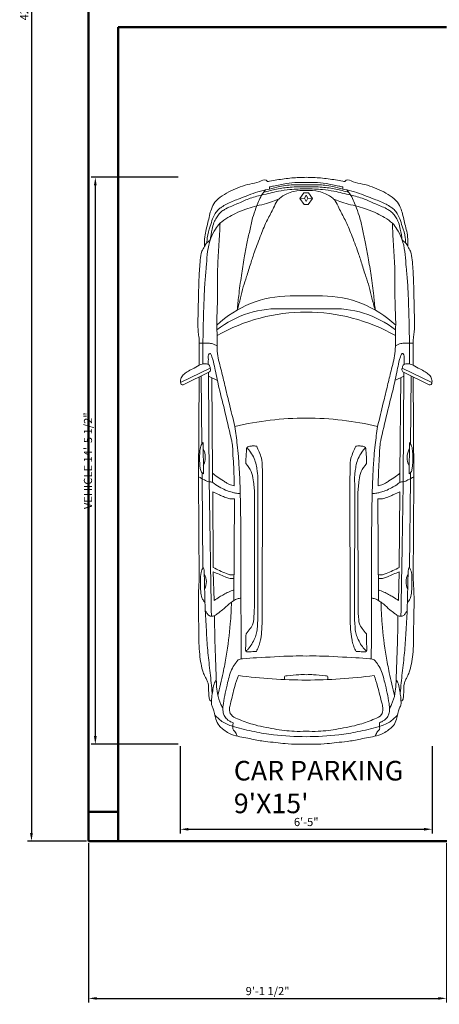
# Model space of a CAD drawing. Units: inches. Extents: x 20697 to 21575, y 6189 to 6822.
# Tile 1 of 7: x 20697 to 20826, y 6189 to 6490. Entities that reach past the tile are written whole.
import ezdxf

# ---------------------------------------------------------------- set-up
doc = ezdxf.new("R2010")
doc.units = ezdxf.units.IN
for name, color, linetype, lineweight in [('A-ANNO-DIMS', 2, 'Continuous', 18), ('A-AREA-IDEN', 7, 'Continuous', 18), ('A-SITE-VEHC', 8, 'Continuous', 13), ('A-WALL', 7, 'Continuous', 50)]:
    doc.layers.add(name, color=color, linetype=linetype, lineweight=lineweight)
doc.styles.get("Standard").update_dxf_attribs({"font": 'arial.ttf'})
doc.dimstyles.new('ISO-25', dxfattribs={"dimtxt": 2.5, "dimasz": 2.5, "dimexe": 1.25, "dimexo": 0.625, "dimtad": 1, "dimdec": 0, "dimlunit": 3, "dimtxsty": 'Standard', "dimcen": 2.5, "dimadec": 0, "dimazin": 0, "dimtfac": 1, "dimtdec": 0, "dimtmove": 0, "dimatfit": 3, "dimfxl": 1, "dimarcsym": 0})

# ---------------------------------------------------------------- blocks, each defined once
blk = doc.blocks.new('*D6')
at = {"layer": 'A-ANNO-DIMS', "color": 0, "lineweight": -2, "transparency": 16777216}
for p, q in [((20717.67, 6750.06), (20699.54, 6750.06)), ((20700.79, 6747.56), (20700.79, 6241.06)), ((20717.67, 6238.56), (20699.54, 6238.56))]:
    blk.add_line(p, q, dxfattribs=at)
at = {"layer": 'A-ANNO-DIMS', "color": 0, "transparency": 16777216}
for points in [[(20700.37, 6747.56), (20701.21, 6747.56), (20700.79, 6750.06)], [(20700.37, 6241.06), (20701.21, 6241.06), (20700.79, 6238.56)]]:
    blk.add_solid(points, dxfattribs=at)
at = {"layer": 'Defpoints', "color": 0, "transparency": 16777216}
for p in [(20718.29, 6750.06), (20700.79, 6238.56), (20718.29, 6238.56)]:
    blk.add_point(p, dxfattribs=at)
at = {"layer": 'A-ANNO-DIMS', "color": 0, "transparency": 16777216, "insert": (20698.89, 6494.31), "char_height": 2.5, "attachment_point": 5, "rotation": 90}
blk.add_mtext('42\'-8"', dxfattribs=at)
blk = doc.blocks.new('A$C37D034A9')
for p, q in [((1532.9, 1782), (1646.8, 2021.3)), ((1562, 1787.5), (1667.1, 1999.6)), ((1303.4, 1869.8), (1509.9, 1870.9)), ((1332.7, 1840.6), (1499.3, 1841.7)), ((1594.8, 1853.7), (2145, 1849.8)), ((1603.5, 1871.3), (2420.8, 1875.4)), ((2129.3, 1839.6), (2381.5, 1836.9)), ((2373.8, 1848.2), (2422.4, 1847.8)), ((2420.8, 1875.4), (3234.3, 1871.4)), ((2422.4, 1847.8), (3133.1, 1841.3)), ((3158, 1831.3), (3479.6, 1822.1)), ((1565.9, 1795.4), (2445.8, 1790.4)), ((1632.4, 1724.1), (1596.5, 1795.2)), ((2377.3, 1763.7), (1609.3, 1769.9)), ((2377.3, 1763.7), (2449.6, 1763.3)), ((2525, 1762.2), (3132.5, 1759)), ((3168.1, 1757.9), (3399.7, 1751.2)), ((2582.7, 1587), (3399.6, 1592.9)), ((2539.6, 1425.8), (3453, 1427.6)), ((2405.7, 1362.6), (3533.3, 1364.3)), ((2458.8, 1400.3), (3499.1, 1398.6)), ((76.9, 1306.3), (96.6, 1306.3)), ((96.6, 1306.3), (101.3, 1337.1)), ((952, 1010.8), (952, 1141.1)), ((1057.1, 1010.8), (1057.1, 1185.6)), ((124.1, 1010.8), (124.7, 1029.9)), ((124.7, 1029.9), (169.4, 1060.8)), ((169.4, 1060.8), (168.8, 1024.8)), ((169.4, 1060.8), (219.8, 1027.6)), ((124.1, 1010.8), (124.7, 991.8)), ((124.7, 991.8), (169.4, 960.9)), ((143, 1010.8), (168.8, 1024.8)), ((143, 1010.8), (168.8, 996.9)), ((168.8, 1024.8), (195.2, 1010.8)), ((168.8, 996.9), (195.2, 1010.8)), ((169.4, 960.9), (168.8, 996.9)), ((169.4, 960.9), (219.8, 994.1)), ((219.8, 1027.6), (219.8, 1010.8)), ((219.8, 994.1), (219.8, 1010.8)), ((952, 1010.8), (952, 880.6)), ((1057.1, 1010.8), (1057.1, 836.1)), ((76.9, 715.4), (96.6, 715.4)), ((96.6, 715.4), (101.3, 684.5)), ((2405.7, 659.1), (3533.3, 657.4)), ((2458.8, 621.4), (3499.1, 623.1)), ((2539.6, 595.9), (3453, 594.1)), ((2582.7, 434.7), (3399.6, 428.8)), ((1532.9, 239.7), (1646.8, 0.4)), ((1632.4, 297.6), (1596.5, 226.5)), ((2377.3, 258), (1609.3, 251.8)), ((2377.3, 258), (2449.6, 258.4)), ((2525, 259.5), (3132.5, 262.7)), ((3168.1, 263.8), (3399.7, 270.5)), ((1332.7, 181), (1499.3, 180)), ((1562, 234.2), (1667.1, 22.1)), ((1565.9, 226.3), (2445.8, 231.3)), ((1594.8, 168), (2145, 171.9)), ((2129.3, 182.1), (2381.5, 184.7)), ((2373.8, 173.5), (2422.4, 173.9)), ((2422.4, 173.9), (3133.1, 180.4)), ((3158, 190.4), (3479.6, 199.6)), ((1303.4, 151.9), (1509.9, 150.8)), ((1603.5, 150.4), (2420.8, 146.3)), ((2420.8, 146.3), (3234.3, 150.3))]:
    blk.add_line(p, q)
for centre, radius, start, end in [((2249.9, 1966.9), 145.3, 241.65089, 297.15378), ((3250.7, 1930.2), 117.1, 238.4977, 298.20211), ((1820.6, 1134.2), 868.6, 136.71033, 179.54402), ((1853.1, 1235.9), 797.6, 141.87926, 183.61449), ((2543.6, 1010.3), 1461.1, 150.60457, 179.97848), ((4391.3, 1012.9), 2457.7, 166.55485, 180.04792), ((-73, 1011.6), 4110.5, 359.98923, 7.61333), ((2543.6, 1011.4), 1461.1, 180.02152, 209.39543), ((4391.3, 1008.8), 2457.7, 179.95208, 193.44515), ((-73, 1010.1), 4110.5, 352.38667, 0.01077), ((1820.6, 887.5), 868.6, 180.45598, 223.28967), ((1853.1, 785.8), 797.6, 176.38551, 218.12074), ((2249.9, 54.7), 145.3, 62.84622, 118.34911), ((3250.7, 91.5), 117.1, 61.79789, 121.5023)]:
    blk.add_arc(centre, radius, start, end)
for points, knots in [([(1526.7, 1783.8), (1518.5, 1785.4), (1502.6, 1788.6), (1494, 1821.1), (1503, 1863.1), (1531.4, 1908.3), (1553.6, 1954.9), (1577.5, 1992.7), (1609, 2018.2), (1639.6, 2023.8), (1665.5, 2017.7), (1667.4, 2005.2), (1667.1, 1999.6)], [0, 0, 0, 0, 0.0238674, 0.0459576, 0.0928721, 0.1559652, 0.2092168, 0.2528802, 0.29396, 0.3295755, 0.3493177, 0.3652101, 0.3652101, 0.3652101, 0.3652101]), ([(0, 1010.8), (0.9, 1049.4), (2.7, 1128.2), (18.7, 1227.6), (27.1, 1289.4), (36.3, 1321.4), (9.1, 1341.9), (46.5, 1397.5), (51.1, 1463.8), (76, 1541.9), (106.6, 1616.4), (147, 1685.7), (193.4, 1744.6), (269.5, 1782.5), (364.9, 1798.9), (463.9, 1829.1), (529.8, 1828.6), (556.4, 1828.4)], [0, 0, 0, 0, 115.859327, 237.079713, 296.141984, 312.044705, 327.106088, 383.833978, 461.944264, 541.76825, 623.45364, 704.555207, 782.226587, 843.70687, 954.283591, 1071.961262, 1151.295838, 1151.295838, 1151.295838, 1151.295838]), ([(171.7, 1228.4), (179.9, 1245.7), (198.1, 1284.1), (217.3, 1351.6), (232.9, 1424.6), (256.4, 1502.6), (284.7, 1575), (325.4, 1642.9), (361.7, 1702.7), (421.9, 1744.6), (473.5, 1772.8), (542.2, 1795.2), (621.2, 1808), (729.6, 1813.6), (852.5, 1827.6), (985.4, 1831.9), (1147.8, 1837.9), (1262.1, 1839.6), (1332.7, 1840.6)], [0, 0, 0, 0, 57.118397, 127.539793, 209.532187, 281.268626, 371.866644, 441.418243, 519.229725, 578.070076, 658.62539, 694.988053, 794.237238, 897.694875, 1020.566778, 1165.110139, 1296.310821, 1508.108184, 1508.108184, 1508.108184, 1508.108184]), ([(505.9, 1783.2), (511.7, 1792.2), (524.3, 1811.9), (558.6, 1828.8), (601.3, 1855.8), (687.8, 1865.5), (801.6, 1872.4), (931.7, 1876.4), (1052.9, 1878.6), (1152.2, 1881.4), (1229.2, 1880.7), (1271.8, 1874.5), (1295.8, 1871.8), (1303.4, 1869.8)], [0, 0, 0, 0, 0.0326993, 0.0711104, 0.1154542, 0.1883548, 0.3342533, 0.4716751, 0.5906313, 0.709353, 0.7812775, 0.8251283, 0.8483376, 0.8483376, 0.8483376, 0.8483376]), ([(1352.2, 1727.5), (1348.6, 1734.7), (1341.5, 1749.1), (1334, 1774.3), (1330.6, 1801.2), (1331.6, 1824.1), (1333.2, 1846.5), (1333.1, 1860.1), (1333, 1869.8)], [0, 0, 0, 0, 24.224889, 47.981341, 78.378061, 105.14947, 116.640041, 145.779732, 145.779732, 145.779732, 145.779732]), ([(2129.3, 1839.6), (2139.3, 1846.4), (2162.1, 1861.8), (2229.8, 1868.5), (2295.3, 1869), (2349.6, 1860.8), (2371.7, 1853), (2377.9, 1842.9), (2381.5, 1836.9)], [0, 0, 0, 0, 35.825501, 81.320865, 199.176406, 232.541501, 246.984194, 267.031211, 267.031211, 267.031211, 267.031211]), ([(2539.5, 1541.1), (2539.2, 1554), (2538.6, 1576.3), (2528.3, 1611.8), (2517, 1652), (2491.9, 1699.9), (2471, 1739.2), (2444.9, 1765.9), (2448.6, 1796.4), (2428.8, 1832.5), (2413.3, 1859.8), (2404.6, 1875.3)], [0, 0, 0, 0, 38.745445, 66.586145, 110.33194, 163.856449, 227.516292, 245.160425, 271.043315, 311.933858, 365.718129, 365.718129, 365.718129, 365.718129]), ([(3133.1, 1841.3), (3146.7, 1846.9), (3179.9, 1860.4), (3247.3, 1860.4), (3314.2, 1860.4), (3370.1, 1853.2), (3398.7, 1838.7), (3410.3, 1828.3), (3415.2, 1823.9)], [0, 0, 0, 0, 43.951201, 106.610136, 198.707081, 246.448273, 273.585601, 293.13086, 293.13086, 293.13086, 293.13086]), ([(3133.1, 1841.3), (3135, 1839.5), (3139.3, 1835.5), (3148, 1831.9), (3154.6, 1831.5), (3158, 1831.3)], [0, 0, 0, 0, 7.956866, 17.272723, 27.586643, 27.586643, 27.586643, 27.586643]), ([(3234.3, 1871.4), (3278.5, 1873.9), (3359.8, 1878.7), (3498.2, 1876.9), (3652.8, 1872.6), (3796.5, 1873.5), (3904.8, 1856.8), (3965.7, 1843.6), (4008.7, 1824.5), (4036.7, 1808.6), (4079.2, 1792.4), (4128.2, 1796.5), (4172.2, 1791.8), (4202.5, 1788.4), (4205.6, 1775.1), (4206.3, 1771.9)], [0, 0, 0, 0, 132.674859, 244.267951, 415.033268, 597.210204, 673.623963, 743.864874, 783.070086, 814.193218, 840.469708, 918.651615, 953.206586, 982.809878, 992.270601, 992.270601, 992.270601, 992.270601]), ([(3379.8, 1535.3), (3380.7, 1545.1), (3382.7, 1565.9), (3401.9, 1597.3), (3430.4, 1638), (3469.9, 1676.8), (3498.2, 1716.6), (3521, 1743.8), (3525.9, 1769.6), (3522.3, 1795.4), (3500.7, 1808.9), (3486.5, 1817.7), (3479.6, 1822.1)], [0, 0, 0, 0, 29.359586, 61.637967, 108.210927, 179.145324, 226.057178, 255.76704, 283.158676, 303.178471, 328.962154, 354.067963, 354.067963, 354.067963, 354.067963]), ([(3479.6, 1822.1), (3538.8, 1818.8), (3651.5, 1812.5), (3818.6, 1802.2), (3979.7, 1781.5), (4087.9, 1771.6), (4142.1, 1766.6)], [0, 0, 0, 0, 177.941766, 338.827113, 501.856877, 665.021059, 665.021059, 665.021059, 665.021059]), ([(101.3, 1337.1), (107.8, 1364.5), (120.6, 1417.6), (150.6, 1489.5), (178.2, 1568.8), (207.7, 1635.1), (236.1, 1688.4), (260.7, 1718.9), (292, 1744.4), (337.6, 1766.1), (403.7, 1784.8), (466.8, 1807.4), (512, 1808.2), (525.1, 1808.4)], [0, 0, 0, 0, 84.171622, 163.614553, 233.045723, 336.213067, 381.194856, 413.584235, 453.241792, 501.082694, 563.744046, 659.867603, 698.986252, 698.986252, 698.986252, 698.986252]), ([(142.1, 1367.1), (151.1, 1402.9), (168, 1470.3), (214.3, 1562.8), (239.3, 1634.9), (268.9, 1683.6), (292.1, 1711.1), (325.5, 1734.1), (365.7, 1755.6), (427.7, 1769.9), (475.9, 1778.1), (505.9, 1783.2)], [0, 0, 0, 0, 110.301969, 207.85498, 309.529413, 337.706505, 378.588004, 416.258758, 458.790096, 514.345906, 605.771135, 605.771135, 605.771135, 605.771135]), ([(1500.6, 1799.3), (1483.6, 1797.8), (1458.3, 1795.7), (1428.9, 1799.6), (1404, 1781.1), (1466.2, 1759.6), (1531.4, 1744.8), (1686.1, 1714.1), (1872.2, 1665.2), (2027.8, 1629.7), (2149.6, 1601.2), (2228.7, 1601.2), (2331, 1591.7), (2412.2, 1590.6), (2462.2, 1589.4), (2477.9, 1589.1)], [0, 0, 0, 0, 50.83029, 75.434549, 89.950931, 122.622478, 199.812772, 348.247849, 559.911218, 792.840685, 822.965183, 934.929309, 1028.100235, 1131.331462, 1178.338034, 1178.338034, 1178.338034, 1178.338034]), ([(1562, 1787.5), (1559.1, 1784.6), (1548.4, 1777.2), (1535.5, 1781.2), (1526.6, 1783.9)], [0.60973338, 0.60973338, 0.60973338, 0.60973338, 0.62203277, 0.64851229, 0.64851229, 0.64851229, 0.64851229]), ([(2477.9, 1589.1), (2475, 1602.1), (2470.4, 1622.6), (2455.4, 1651.1), (2432.7, 1682.8), (2408.1, 1722.8), (2386.6, 1751.4), (2377.3, 1763.7)], [0, 0, 0, 0, 39.93807, 62.488042, 96.043823, 157.027531, 203.188279, 203.188279, 203.188279, 203.188279]), ([(2445.8, 1790.4), (2667.6, 1786.9), (3027.2, 1781.3), (3386.8, 1774.8), (3524.6, 1772.4)], [0, 0, 0, 0, 665.499287, 1078.912831, 1078.912831, 1078.912831, 1078.912831]), ([(2582.7, 1587), (2583.2, 1597), (2584.1, 1618.1), (2575.7, 1651.7), (2561.4, 1682.9), (2545.4, 1721), (2533, 1746.1), (2525, 1762.2)], [0, 0, 0, 0, 29.813022, 63.072982, 102.549857, 133.014078, 186.71332, 186.71332, 186.71332, 186.71332]), ([(3190.5, 1591.4), (3191.8, 1602.2), (3194.2, 1623.2), (3178.9, 1661.6), (3159.5, 1706.6), (3141.5, 1741.5), (3132.5, 1759)], [0, 0, 0, 0, 32.129278, 62.428148, 121.529201, 180.173044, 180.173044, 180.173044, 180.173044]), ([(3221.3, 1591.6), (3222.3, 1599.2), (3224.2, 1612.8), (3218.1, 1637.1), (3198.8, 1684.5), (3181.3, 1726.4), (3168.1, 1757.9)], [0, 0, 0, 0, 22.895094, 40.749622, 74.16608, 176.695684, 176.695684, 176.695684, 176.695684]), ([(3399.7, 1751.2), (3389.2, 1737.2), (3370.8, 1712.4), (3351.4, 1671.7), (3328.3, 1635.1), (3318.4, 1607), (3313.2, 1592.2)], [0, 0, 0, 0, 52.277284, 92.404872, 134.765704, 181.565756, 181.565756, 181.565756, 181.565756]), ([(3520.4, 1748.4), (3581.5, 1747.4), (3690.9, 1745.6), (3850.5, 1740.6), (3997.8, 1733.6), (4128.7, 1732.6), (4218, 1705.9), (4256.1, 1686.1), (4266.8, 1680.5)], [0, 0, 0, 0, 0.1893068, 0.338908, 0.4944806, 0.646686, 0.7418914, 0.7794792, 0.7794792, 0.7794792, 0.7794792]), ([(4034.2, 1733.6), (4045.8, 1740.2), (4074.3, 1756.4), (4123, 1760.8), (4168.2, 1770.9), (4204, 1771), (4235.2, 1775.6), (4280.4, 1748.5), (4340.7, 1743.1), (4401.4, 1717.8), (4431.8, 1679.8), (4465, 1638.3), (4492.9, 1557.6), (4508.3, 1454.7), (4532.6, 1348.3), (4538.1, 1258.3), (4550, 1171.3), (4553.1, 1089.6), (4552.8, 1033), (4552.7, 1010.8)], [0, 0, 0, 0, 39.653141, 97.537887, 144.067219, 178.030901, 205.682198, 235.219107, 329.899318, 386.728403, 425.383384, 473.826134, 545.717065, 677.079425, 786.867362, 871.982002, 947.184951, 1050.283917, 1116.835862, 1116.835862, 1116.835862, 1116.835862]), ([(4319.3, 1743.9), (4339.8, 1723.4), (4383.7, 1679.5), (4421.6, 1566.1), (4452, 1430.6), (4487, 1238.2), (4490.2, 1098.7), (4492.3, 1010.8)], [0, 0, 0, 0, 85.725408, 184.11518, 350.578699, 505.359156, 768.57646, 768.57646, 768.57646, 768.57646]), ([(368.8, 1703.1), (425.1, 1705.7), (540.8, 1711), (717, 1724.8), (900.9, 1721.8), (1058.4, 1725.6), (1167.5, 1731.4), (1251.8, 1726.5), (1327.3, 1728.4), (1438.6, 1725.6), (1547.2, 1692.8), (1679.5, 1663), (1828.2, 1626.4), (1937.8, 1599.7), (2000.9, 1584.4)], [0, 0, 0, 0, 169.036427, 347.362971, 529.912023, 720.398665, 820.073141, 857.414524, 973.264583, 1046.863942, 1190.103596, 1310.627442, 1454.37964, 1649.234994, 1649.234994, 1649.234994, 1649.234994]), ([(3411.7, 1610.9), (3469.8, 1613.6), (3614.8, 1620.2), (3804, 1644.2), (3995.7, 1680.7), (4101, 1706), (4162.1, 1720.6)], [0, 0, 0, 0, 174.545563, 435.159645, 571.339835, 759.876078, 759.876078, 759.876078, 759.876078]), ([(4380.1, 1598.9), (4377.5, 1605.6), (4372, 1620.1), (4356.9, 1644.3), (4333.4, 1666.4), (4303.5, 1677.7), (4268.1, 1682), (4185.7, 1672.3), (4075, 1646.1), (3959.1, 1618.7), (3904, 1580.2), (3870.2, 1557), (3862, 1494.9), (3857.6, 1352), (3843.1, 1179.6), (3844.2, 1046.6), (3844.5, 1010.8)], [0, 0, 0, 0, 21.644576, 46.330939, 85.252079, 115.796407, 140.70863, 191.639103, 362.713195, 485.636819, 539.797523, 566.31637, 603.271258, 715.496747, 1007.274347, 1114.772665, 1114.772665, 1114.772665, 1114.772665]), ([(2000.9, 1584.4), (2050.2, 1577.5), (2130.3, 1566.4), (2257.3, 1554.3), (2428.3, 1543.9), (2677.9, 1536.6), (3173.5, 1535.9), (3575.5, 1534.8), (3868.2, 1533.9)], [0, 0, 0, 0, 149.160554, 242.516206, 382.750296, 663.136182, 991.365177, 1869.419131, 1869.419131, 1869.419131, 1869.419131]), ([(4001.2, 1556.2), (4030.1, 1566.1), (4104.8, 1591.8), (4195.3, 1610.4), (4270.6, 1631.7), (4325, 1618.5), (4359.2, 1540.1), (4400.9, 1427.7), (4430.3, 1273), (4451.3, 1129.1), (4449.5, 1043.2), (4448.8, 1010.8)], [0, 0, 0, 0, 91.386952, 236.7281, 276.8874, 325.656701, 388.160417, 515.845838, 694.439347, 855.118843, 951.905721, 951.905721, 951.905721, 951.905721]), ([(4487.8, 1564.7), (4478.2, 1568.8), (4462.1, 1575.6), (4445.4, 1588.5), (4432, 1603.7), (4407.3, 1599.2), (4389.6, 1599), (4380.1, 1598.9)], [0, 0, 0, 0, 31.069852, 51.968535, 63.635964, 88.937852, 118.267317, 118.267317, 118.267317, 118.267317]), ([(101.3, 1337.1), (115.6, 1348.3), (144.8, 1371.1), (195.1, 1395.5), (256.3, 1417.7), (333.1, 1446.5), (429.6, 1464.1), (535.3, 1489.3), (655.2, 1511.3), (795.4, 1533), (935.6, 1552.1), (1028.3, 1561.3), (1066.4, 1565.1)], [0, 0, 0, 0, 54.341871, 110.809469, 166.465422, 250.120596, 356.027662, 459.965647, 576.273716, 721.357641, 885.82263, 1000.664546, 1000.664546, 1000.664546, 1000.664546]), ([(106.6, 1010.8), (105.7, 1045.1), (104.2, 1099.1), (135.5, 1169.8), (158.1, 1216.7), (197.9, 1253.2), (259.9, 1278), (346.4, 1328.5), (466.2, 1376.7), (582.7, 1421.8), (696.4, 1458.7), (790.2, 1487.4), (881.1, 1518.1), (971.9, 1538.1), (1033.6, 1555.7), (1066.4, 1565.1)], [0, 0, 0, 0, 100.900035, 159.133916, 230.081698, 254.424499, 319.300609, 427.621894, 555.335452, 705.414693, 802.817368, 913.804918, 999.761827, 1090.195484, 1192.415586, 1192.415586, 1192.415586, 1192.415586]), ([(2298, 1495.5), (2274, 1495.3), (2236.7, 1495), (2196, 1490.4), (2168.6, 1489.4), (2160.2, 1467.6), (2156.5, 1442), (2158, 1420.5), (2158.9, 1408.7)], [0, 0, 0, 0, 71.046649, 110.558827, 128.37963, 144.71322, 173.076989, 208.45657, 208.45657, 208.45657, 208.45657]), ([(2170.3, 1486.3), (2182.7, 1476.3), (2210, 1454.2), (2256.4, 1428.5), (2306.5, 1411.4), (2351.9, 1405.7), (2401.7, 1398.2), (2436.4, 1399.5), (2458.8, 1400.3)], [0, 0, 0, 0, 47.797708, 105.289438, 158.269533, 205.372846, 242.305865, 309.191827, 309.191827, 309.191827, 309.191827]), ([(2298, 1495.5), (2318.7, 1479.3), (2358, 1448.6), (2443.9, 1432.4), (2503.4, 1428.3), (2539.6, 1425.8)], [0, 0, 0, 0, 77.358827, 147.491986, 256.835629, 256.835629, 256.835629, 256.835629]), ([(3453, 1427.6), (3486.4, 1428.6), (3530.4, 1429.9), (3589.9, 1436.8), (3627, 1462.3), (3652.8, 1482.8), (3667.2, 1494.2)], [0, 0, 0, 0, 100.486425, 132.77915, 176.765793, 232.152339, 232.152339, 232.152339, 232.152339]), ([(3499.1, 1398.6), (3536.1, 1399.2), (3589.3, 1400.2), (3657.1, 1407.8), (3703.6, 1424), (3747.4, 1446.7), (3783.3, 1471.1), (3799.9, 1489.6), (3805.4, 1495.7)], [0, 0, 0, 0, 111.072131, 159.897362, 203.565673, 257.821021, 307.92378, 332.338193, 332.338193, 332.338193, 332.338193]), ([(3667.2, 1494.2), (3685.9, 1495.1), (3724, 1496.8), (3766.2, 1495.9), (3817.3, 1501.3), (3808.3, 1449.9), (3808.3, 1423.8), (3808.2, 1411.3)], [0, 0, 0, 0, 55.464151, 112.394664, 138.340379, 182.296823, 222.9909, 222.9909, 222.9909, 222.9909]), ([(75.3, 1010.8), (76, 1053.5), (77.3, 1133.2), (91.8, 1247.9), (111.2, 1317.8), (120.7, 1352.1)], [0, 0, 0, 0, 128.021764, 238.88679, 345.525832, 345.525832, 345.525832, 345.525832]), ([(92.6, 1010.8), (93.4, 1054.5), (94.8, 1129.2), (108.9, 1226), (126.9, 1300.5), (137, 1344.9), (142.1, 1367.1)], [0, 0, 0, 0, 130.850655, 223.863722, 292.648971, 360.733198, 360.733198, 360.733198, 360.733198]), ([(2158.9, 1408.7), (2174.5, 1402.1), (2206.5, 1388.8), (2261.1, 1365.4), (2329.9, 1363.2), (2379.8, 1362.8), (2405.7, 1362.6)], [0, 0, 0, 0, 50.927539, 104.178585, 176.434127, 254.369734, 254.369734, 254.369734, 254.369734]), ([(3533.3, 1364.3), (3566.3, 1364.8), (3623.8, 1365.6), (3695.2, 1374), (3747.6, 1385.7), (3781.9, 1398), (3801.7, 1408), (3808.2, 1411.3)], [0, 0, 0, 0, 98.831069, 172.48171, 215.199389, 259.51023, 281.524611, 281.524611, 281.524611, 281.524611]), ([(41.8, 1010.8), (41.2, 1033.5), (39.6, 1087.1), (45.9, 1157.9), (61.8, 1221.8), (69.7, 1267), (74.9, 1295.4), (76.9, 1306.3)], [0, 0, 0, 0, 67.884516, 160.875373, 212.043403, 265.217267, 298.518591, 298.518591, 298.518591, 298.518591]), ([(59.3, 1010.8), (59.3, 1041.9), (59.2, 1092.1), (63, 1164.1), (75.5, 1231.8), (89, 1279.6), (96.6, 1306.3)], [0, 0, 0, 0, 93.279537, 150.555964, 216.000548, 299.30356, 299.30356, 299.30356, 299.30356]), ([(3994.3, 1010.8), (3993.8, 1030.5), (3992.7, 1082.7), (4001.7, 1133.4), (4004.3, 1188.4), (4022.7, 1184.7), (4033.9, 1182.4)], [0, 0, 0, 0, 58.064484, 154.084598, 171.257643, 198.43549, 198.43549, 198.43549, 198.43549]), ([(0, 1010.8), (0.9, 972.3), (2.7, 893.5), (18.7, 794.1), (27.1, 732.3), (36.3, 700.3), (9.1, 679.8), (46.5, 624.2), (51.1, 557.8), (76, 479.8), (106.6, 405.3), (147, 336), (193.4, 277.1), (269.5, 239.2), (364.9, 222.8), (463.9, 192.6), (529.8, 193.1), (556.4, 193.2)], [0, 0, 0, 0, 115.859327, 237.079713, 296.141984, 312.044705, 327.106088, 383.833978, 461.944264, 541.76825, 623.45364, 704.555207, 782.226587, 843.70687, 954.283591, 1071.961262, 1151.295838, 1151.295838, 1151.295838, 1151.295838]), ([(41.8, 1010.8), (41.2, 988.2), (39.6, 934.6), (45.9, 863.8), (61.8, 799.9), (69.7, 754.7), (74.9, 726.3), (76.9, 715.4)], [0, 0, 0, 0, 67.884516, 160.875373, 212.043403, 265.217267, 298.518591, 298.518591, 298.518591, 298.518591]), ([(59.3, 1010.8), (59.3, 979.8), (59.2, 929.6), (63, 857.6), (75.5, 789.9), (89, 742.1), (96.6, 715.4)], [0, 0, 0, 0, 93.279537, 150.555964, 216.000548, 299.30356, 299.30356, 299.30356, 299.30356]), ([(75.3, 1010.8), (76, 968.2), (77.3, 888.5), (91.8, 773.8), (111.2, 703.9), (120.7, 669.6)], [0, 0, 0, 0, 128.021764, 238.88679, 345.525832, 345.525832, 345.525832, 345.525832]), ([(92.6, 1010.8), (93.4, 967.2), (94.8, 892.5), (108.9, 795.7), (126.9, 721.2), (137, 676.8), (142.1, 654.6)], [0, 0, 0, 0, 130.850655, 223.863722, 292.648971, 360.733198, 360.733198, 360.733198, 360.733198]), ([(106.6, 1010.8), (105.7, 976.6), (104.2, 922.6), (135.5, 851.9), (158.1, 805), (197.9, 768.5), (259.9, 743.7), (346.4, 693.2), (466.2, 645), (582.7, 599.9), (696.4, 563), (790.2, 534.3), (881.1, 503.6), (971.9, 483.6), (1033.6, 465.9), (1066.4, 456.6)], [0, 0, 0, 0, 100.900035, 159.133916, 230.081698, 254.424499, 319.300609, 427.621894, 555.335452, 705.414693, 802.817368, 913.804918, 999.761827, 1090.195484, 1192.415586, 1192.415586, 1192.415586, 1192.415586]), ([(4380.1, 422.8), (4377.5, 416.1), (4372, 401.6), (4356.9, 377.4), (4333.4, 355.3), (4303.5, 344), (4268.1, 339.7), (4185.7, 349.4), (4075, 375.6), (3959.1, 403), (3904, 441.5), (3870.2, 464.7), (3862, 526.8), (3857.6, 669.7), (3843.1, 842.1), (3844.2, 975.1), (3844.5, 1010.8)], [0, 0, 0, 0, 21.644576, 46.330939, 85.252079, 115.796407, 140.70863, 191.639103, 362.713195, 485.636819, 539.797523, 566.31637, 603.271258, 715.496747, 1007.274347, 1114.772665, 1114.772665, 1114.772665, 1114.772665]), ([(3994.3, 1010.8), (3993.8, 991.2), (3992.7, 939), (4001.7, 888.3), (4004.3, 833.3), (4022.7, 837), (4033.9, 839.3)], [0, 0, 0, 0, 58.064484, 154.084598, 171.257643, 198.43549, 198.43549, 198.43549, 198.43549]), ([(4001.2, 465.5), (4030.1, 455.6), (4104.8, 429.9), (4195.3, 411.3), (4270.6, 390), (4325, 403.2), (4359.2, 481.6), (4400.9, 594), (4430.3, 748.7), (4451.3, 892.6), (4449.5, 978.5), (4448.8, 1010.8)], [0, 0, 0, 0, 91.386952, 236.7281, 276.8874, 325.656701, 388.160417, 515.845838, 694.439347, 855.118843, 951.905721, 951.905721, 951.905721, 951.905721]), ([(4034.2, 288), (4045.8, 281.5), (4074.3, 265.3), (4123, 260.9), (4168.2, 250.8), (4204, 250.7), (4235.2, 246.1), (4280.4, 273.2), (4340.7, 278.6), (4401.4, 303.9), (4431.8, 341.9), (4465, 383.4), (4492.9, 464.1), (4508.3, 567), (4532.6, 673.4), (4538.1, 763.4), (4550, 850.4), (4553.1, 932.1), (4552.8, 988.7), (4552.7, 1010.8)], [0, 0, 0, 0, 39.653141, 97.537887, 144.067219, 178.030901, 205.682198, 235.219107, 329.899318, 386.728403, 425.383384, 473.826134, 545.717065, 677.079425, 786.867362, 871.982002, 947.184951, 1050.283917, 1116.835862, 1116.835862, 1116.835862, 1116.835862]), ([(4319.3, 277.8), (4339.8, 298.3), (4383.7, 342.2), (4421.6, 455.6), (4452, 591.1), (4487, 783.5), (4490.2, 923), (4492.3, 1010.8)], [0, 0, 0, 0, 85.725408, 184.11518, 350.578699, 505.359156, 768.57646, 768.57646, 768.57646, 768.57646]), ([(171.7, 793.2), (179.9, 776), (198.1, 737.6), (217.3, 670.1), (232.9, 597.1), (256.4, 519.1), (284.7, 446.7), (325.4, 378.8), (361.7, 319), (421.9, 277.1), (473.5, 248.9), (542.2, 226.5), (621.2, 213.7), (729.6, 208.1), (852.5, 194.1), (985.4, 189.8), (1147.8, 183.8), (1262.1, 182.1), (1332.7, 181)], [0, 0, 0, 0, 57.118397, 127.539793, 209.532187, 281.268626, 371.866644, 441.418243, 519.229725, 578.070076, 658.62539, 694.988053, 794.237238, 897.694875, 1020.566778, 1165.110139, 1296.310821, 1508.108184, 1508.108184, 1508.108184, 1508.108184]), ([(101.3, 684.5), (107.8, 657.2), (120.6, 604.1), (150.6, 532.2), (178.2, 452.9), (207.7, 386.5), (236.1, 333.3), (260.7, 302.8), (292, 277.3), (337.6, 255.6), (403.7, 236.9), (466.8, 214.3), (512, 213.5), (525.1, 213.3)], [0, 0, 0, 0, 84.171622, 163.614553, 233.045723, 336.213067, 381.194856, 413.584235, 453.241792, 501.082694, 563.744046, 659.867603, 698.986252, 698.986252, 698.986252, 698.986252]), ([(101.3, 684.5), (115.6, 673.4), (144.8, 650.6), (195.1, 626.2), (256.3, 604), (333.1, 575.2), (429.6, 557.6), (535.3, 532.4), (655.2, 510.4), (795.4, 488.7), (935.6, 469.6), (1028.3, 460.4), (1066.4, 456.6)], [0, 0, 0, 0, 54.341871, 110.809469, 166.465422, 250.120596, 356.027662, 459.965647, 576.273716, 721.357641, 885.82263, 1000.664546, 1000.664546, 1000.664546, 1000.664546]), ([(142.1, 654.6), (151.1, 618.8), (168, 551.4), (214.3, 458.9), (239.3, 386.8), (268.9, 338.1), (292.1, 310.6), (325.5, 287.6), (365.7, 266.1), (427.7, 251.8), (475.9, 243.6), (505.9, 238.5)], [0, 0, 0, 0, 110.301969, 207.85498, 309.529413, 337.706505, 378.588004, 416.258758, 458.790096, 514.345906, 605.771135, 605.771135, 605.771135, 605.771135]), ([(2158.9, 613), (2174.5, 619.6), (2206.5, 632.9), (2261.1, 656.3), (2329.9, 658.5), (2379.8, 658.9), (2405.7, 659.1)], [0, 0, 0, 0, 50.927539, 104.178585, 176.434127, 254.369734, 254.369734, 254.369734, 254.369734]), ([(3533.3, 657.4), (3566.3, 656.9), (3623.8, 656.1), (3695.2, 647.7), (3747.6, 636), (3781.9, 623.7), (3801.7, 613.7), (3808.2, 610.4)], [0, 0, 0, 0, 98.831069, 172.48171, 215.199389, 259.51023, 281.524611, 281.524611, 281.524611, 281.524611]), ([(2298, 526.2), (2274, 526.4), (2236.7, 526.7), (2196, 531.3), (2168.6, 532.3), (2160.2, 554.1), (2156.5, 579.7), (2158, 601.1), (2158.9, 613)], [0, 0, 0, 0, 71.046649, 110.558827, 128.37963, 144.71322, 173.076989, 208.45657, 208.45657, 208.45657, 208.45657]), ([(2170.3, 535.4), (2182.7, 545.4), (2210, 567.5), (2256.4, 593.2), (2306.5, 610.3), (2351.9, 616), (2401.7, 623.5), (2436.4, 622.2), (2458.8, 621.4)], [0, 0, 0, 0, 47.797708, 105.289438, 158.269533, 205.372846, 242.305865, 309.191827, 309.191827, 309.191827, 309.191827]), ([(2298, 526.2), (2318.7, 542.4), (2358, 573.1), (2443.9, 589.3), (2503.4, 593.4), (2539.6, 595.9)], [0, 0, 0, 0, 77.358827, 147.491986, 256.835629, 256.835629, 256.835629, 256.835629]), ([(3453, 594.1), (3486.4, 593.1), (3530.4, 591.8), (3589.9, 584.9), (3627, 559.4), (3652.8, 538.9), (3667.2, 527.5)], [0, 0, 0, 0, 100.486425, 132.77915, 176.765793, 232.152339, 232.152339, 232.152339, 232.152339]), ([(3499.1, 623.1), (3536.1, 622.5), (3589.3, 621.5), (3657.1, 613.9), (3703.6, 597.6), (3747.4, 575), (3783.3, 550.6), (3799.9, 532.1), (3805.4, 526)], [0, 0, 0, 0, 111.072131, 159.897362, 203.565673, 257.821021, 307.92378, 332.338193, 332.338193, 332.338193, 332.338193]), ([(3667.2, 527.5), (3685.9, 526.6), (3724, 524.9), (3766.2, 525.8), (3817.3, 520.4), (3808.3, 571.8), (3808.3, 597.9), (3808.2, 610.4)], [0, 0, 0, 0, 55.464151, 112.394664, 138.340379, 182.296823, 222.9909, 222.9909, 222.9909, 222.9909]), ([(2000.9, 437.3), (2050.2, 444.2), (2130.3, 455.3), (2257.3, 467.4), (2428.3, 477.8), (2677.9, 485.1), (3173.5, 485.8), (3575.5, 486.9), (3868.2, 487.8)], [0, 0, 0, 0, 149.160554, 242.516206, 382.750296, 663.136182, 991.365177, 1869.419131, 1869.419131, 1869.419131, 1869.419131]), ([(2539.5, 480.6), (2539.2, 467.7), (2538.6, 445.4), (2528.3, 409.9), (2517, 369.7), (2491.9, 321.8), (2471, 282.5), (2444.9, 255.8), (2448.6, 225.3), (2428.8, 189.2), (2413.3, 161.9), (2404.6, 146.4)], [0, 0, 0, 0, 38.745445, 66.586145, 110.33194, 163.856449, 227.516292, 245.160425, 271.043315, 311.933858, 365.718129, 365.718129, 365.718129, 365.718129]), ([(3379.8, 486.4), (3380.7, 476.5), (3382.7, 455.8), (3401.9, 424.4), (3430.4, 383.7), (3469.9, 344.9), (3498.2, 305.1), (3521, 277.9), (3525.9, 252.1), (3522.3, 226.3), (3500.7, 212.8), (3486.5, 204), (3479.6, 199.6)], [0, 0, 0, 0, 29.359586, 61.637967, 108.210927, 179.145324, 226.057178, 255.76704, 283.158676, 303.178471, 328.962154, 354.067963, 354.067963, 354.067963, 354.067963]), ([(368.8, 318.6), (425.1, 316), (540.8, 310.6), (717, 296.9), (900.9, 299.9), (1058.4, 296.1), (1167.5, 290.3), (1251.8, 295.2), (1327.3, 293.3), (1438.6, 296.1), (1547.2, 328.9), (1679.5, 358.7), (1828.2, 395.3), (1937.8, 422), (2000.9, 437.3)], [0, 0, 0, 0, 169.036427, 347.362971, 529.912023, 720.398665, 820.073141, 857.414524, 973.264583, 1046.863942, 1190.103596, 1310.627442, 1454.37964, 1649.234994, 1649.234994, 1649.234994, 1649.234994]), ([(1500.6, 222.4), (1483.6, 223.9), (1458.3, 226), (1428.9, 222.1), (1404, 240.6), (1466.2, 262.1), (1531.4, 276.9), (1686.1, 307.6), (1872.2, 356.5), (2027.8, 392), (2149.6, 420.5), (2228.7, 420.5), (2331, 430), (2412.2, 431.1), (2462.2, 432.3), (2477.9, 432.6)], [0, 0, 0, 0, 50.83029, 75.434549, 89.950931, 122.622478, 199.812772, 348.247849, 559.911218, 792.840685, 822.965183, 934.929309, 1028.100235, 1131.331462, 1178.338033, 1178.338033, 1178.338033, 1178.338033]), ([(2477.9, 432.6), (2475, 419.6), (2470.4, 399.1), (2455.4, 370.6), (2432.7, 338.9), (2408.1, 298.9), (2386.6, 270.3), (2377.3, 258)], [0, 0, 0, 0, 39.93807, 62.488042, 96.043823, 157.027531, 203.188279, 203.188279, 203.188279, 203.188279]), ([(2582.7, 434.7), (2583.2, 424.7), (2584.1, 403.6), (2575.7, 370), (2561.4, 338.8), (2545.4, 300.7), (2533, 275.6), (2525, 259.5)], [0, 0, 0, 0, 29.813022, 63.072982, 102.549857, 133.014078, 186.71332, 186.71332, 186.71332, 186.71332]), ([(3190.5, 430.3), (3191.8, 419.5), (3194.2, 398.5), (3178.9, 360.1), (3159.5, 315.1), (3141.5, 280.1), (3132.5, 262.7)], [0, 0, 0, 0, 32.129278, 62.428148, 121.529201, 180.173044, 180.173044, 180.173044, 180.173044]), ([(3221.3, 430.1), (3222.3, 422.5), (3224.2, 408.9), (3218.1, 384.6), (3198.8, 337.2), (3181.3, 295.3), (3168.1, 263.8)], [0, 0, 0, 0, 22.895094, 40.749622, 74.16608, 176.695684, 176.695684, 176.695684, 176.695684]), ([(3399.7, 270.5), (3389.2, 284.5), (3370.8, 309.3), (3351.4, 350), (3328.3, 386.6), (3318.4, 414.7), (3313.2, 429.4)], [0, 0, 0, 0, 52.277284, 92.404872, 134.765704, 181.565756, 181.565756, 181.565756, 181.565756]), ([(3411.7, 410.8), (3469.8, 408.1), (3614.8, 401.5), (3804, 377.4), (3995.7, 341), (4101, 315.7), (4162.1, 301)], [0, 0, 0, 0, 174.545563, 435.159645, 571.339835, 759.876078, 759.876078, 759.876078, 759.876078]), ([(4487.8, 457), (4478.2, 452.9), (4462.1, 446.1), (4445.4, 433.2), (4432, 418), (4407.3, 422.5), (4389.6, 422.7), (4380.1, 422.8)], [0, 0, 0, 0, 31.069852, 51.968535, 63.635964, 88.937852, 118.267317, 118.267317, 118.267317, 118.267317]), ([(3520.4, 273.3), (3581.5, 274.3), (3690.9, 276), (3850.5, 281), (3997.8, 288.1), (4128.7, 289.1), (4218, 315.8), (4256.1, 335.6), (4266.8, 341.2)], [0, 0, 0, 0, 0.1893068, 0.338908, 0.4944806, 0.646686, 0.7418914, 0.7794792, 0.7794792, 0.7794792, 0.7794792]), ([(505.9, 238.5), (511.7, 229.5), (524.3, 209.8), (558.6, 192.8), (601.3, 165.9), (687.8, 156.1), (801.6, 149.3), (931.7, 145.3), (1052.9, 143.1), (1152.2, 140.3), (1229.2, 141), (1271.8, 147.1), (1295.8, 149.9), (1303.4, 151.9)], [0, 0, 0, 0, 0.0326993, 0.0711104, 0.1154542, 0.1883548, 0.3342533, 0.4716751, 0.5906313, 0.709353, 0.7812775, 0.8251283, 0.8483376, 0.8483376, 0.8483376, 0.8483376]), ([(1352.2, 294.2), (1348.6, 286.9), (1341.5, 272.6), (1334, 247.4), (1330.6, 220.5), (1331.6, 197.6), (1333.2, 175.2), (1333.1, 161.6), (1333, 151.9)], [0, 0, 0, 0, 24.224889, 47.981341, 78.378061, 105.14947, 116.640041, 145.779732, 145.779732, 145.779732, 145.779732]), ([(1526.7, 237.9), (1518.5, 236.3), (1502.6, 233.1), (1494, 200.6), (1503, 158.6), (1531.4, 113.4), (1553.6, 66.8), (1577.5, 29), (1609, 3.4), (1639.6, -2.1), (1665.5, 4), (1667.4, 16.5), (1667.1, 22.1)], [0, 0, 0, 0, 0.0238674, 0.0459576, 0.0928721, 0.1559652, 0.2092168, 0.2528802, 0.29396, 0.3295755, 0.3493177, 0.3652101, 0.3652101, 0.3652101, 0.3652101]), ([(1562, 234.2), (1559.1, 237.1), (1548.4, 244.5), (1535.5, 240.5), (1526.6, 237.8)], [0.60973338, 0.60973338, 0.60973338, 0.60973338, 0.62203277, 0.64851229, 0.64851229, 0.64851229, 0.64851229]), ([(2445.8, 231.3), (2667.6, 234.8), (3027.2, 240.3), (3386.8, 246.8), (3524.6, 249.3)], [0, 0, 0, 0, 665.499287, 1078.912831, 1078.912831, 1078.912831, 1078.912831]), ([(3234.3, 150.3), (3278.5, 147.8), (3359.8, 143), (3498.2, 144.8), (3652.8, 149), (3796.5, 148.2), (3904.8, 164.9), (3965.7, 178), (4008.7, 197.2), (4036.7, 213.1), (4079.2, 229.2), (4128.2, 225.2), (4172.2, 229.9), (4202.5, 233.3), (4205.6, 246.6), (4206.3, 249.8)], [0, 0, 0, 0, 132.674859, 244.267951, 415.033268, 597.210204, 673.623963, 743.864874, 783.070086, 814.193218, 840.469708, 918.651615, 953.206586, 982.809878, 992.270601, 992.270601, 992.270601, 992.270601]), ([(3479.6, 199.6), (3538.8, 202.9), (3651.5, 209.2), (3818.6, 219.5), (3979.7, 240.2), (4087.9, 250.1), (4142.1, 255.1)], [0, 0, 0, 0, 177.941766, 338.827113, 501.856877, 665.021059, 665.021059, 665.021059, 665.021059]), ([(2129.3, 182.1), (2139.3, 175.3), (2162.1, 159.9), (2229.8, 153.2), (2295.3, 152.7), (2349.6, 160.9), (2371.7, 168.7), (2377.9, 178.8), (2381.5, 184.7)], [0, 0, 0, 0, 35.825501, 81.320865, 199.176406, 232.541501, 246.984194, 267.031211, 267.031211, 267.031211, 267.031211]), ([(3133.1, 180.4), (3146.7, 174.8), (3179.9, 161.3), (3247.3, 161.3), (3314.2, 161.3), (3370.1, 168.5), (3398.7, 183), (3410.3, 193.4), (3415.2, 197.8)], [0, 0, 0, 0, 43.951201, 106.610136, 198.707081, 246.448273, 273.585601, 293.13086, 293.13086, 293.13086, 293.13086]), ([(3133.1, 180.4), (3135, 182.2), (3139.3, 186.2), (3148, 189.8), (3154.6, 190.2), (3158, 190.4)], [0, 0, 0, 0, 7.956866, 17.272723, 27.586643, 27.586643, 27.586643, 27.586643])]:
    blk.add_open_spline(points, degree=3, knots=knots)
blk = doc.blocks.new('*D48')
at = {"layer": 'A-ANNO-DIMS', "color": 0, "lineweight": -2, "transparency": 16777216}
for p, q in [((20745.71, 6441.61), (20719.08, 6441.61)), ((20720.33, 6439.11), (20720.33, 6270.73)), ((20745.71, 6268.23), (20719.08, 6268.23))]:
    blk.add_line(p, q, dxfattribs=at)
at = {"layer": 'A-ANNO-DIMS', "color": 0, "transparency": 16777216}
for points in [[(20719.91, 6439.11), (20720.75, 6439.11), (20720.33, 6441.61)], [(20719.91, 6270.73), (20720.75, 6270.73), (20720.33, 6268.23)]]:
    blk.add_solid(points, dxfattribs=at)
at = {"layer": 'Defpoints', "color": 0, "transparency": 16777216}
for p in [(20746.34, 6441.61), (20720.33, 6268.23), (20746.34, 6268.23)]:
    blk.add_point(p, dxfattribs=at)
at = {"layer": 'A-ANNO-DIMS', "color": 0, "transparency": 16777216, "insert": (20718.41, 6354.92), "char_height": 2.5, "attachment_point": 5, "rotation": 90}
blk.add_mtext('VEHICLE 14\'-5 1/2"', dxfattribs=at)
blk = doc.blocks.new('*D49')
at = {"layer": 'A-ANNO-DIMS', "color": 0, "lineweight": -2, "transparency": 16777216}
for p, q in [((20746.34, 6267.61), (20746.34, 6240.98)), ((20823.4, 6267.61), (20823.4, 6240.98)), ((20748.84, 6242.23), (20820.9, 6242.23))]:
    blk.add_line(p, q, dxfattribs=at)
at = {"layer": 'A-ANNO-DIMS', "color": 0, "transparency": 16777216}
for points in [[(20748.84, 6242.64), (20748.84, 6241.81), (20746.34, 6242.23)], [(20820.9, 6242.64), (20820.9, 6241.81), (20823.4, 6242.23)]]:
    blk.add_solid(points, dxfattribs=at)
at = {"layer": 'Defpoints', "color": 0, "transparency": 16777216}
for p in [(20746.34, 6268.23), (20823.4, 6268.23), (20823.4, 6242.23)]:
    blk.add_point(p, dxfattribs=at)
at = {"layer": 'A-ANNO-DIMS', "color": 0, "transparency": 16777216, "insert": (20784.87, 6244.13), "char_height": 2.5, "attachment_point": 5}
blk.add_mtext('6\'-5"', dxfattribs=at)
blk = doc.blocks.new('*D52')
at = {"layer": 'A-ANNO-DIMS', "color": 0, "lineweight": -2, "transparency": 16777216}
for p, q in [((20718.29, 6237.93), (20718.29, 6189.26)), ((20827.79, 6237.93), (20827.79, 6189.26)), ((20720.79, 6190.51), (20825.29, 6190.51))]:
    blk.add_line(p, q, dxfattribs=at)
at = {"layer": 'A-ANNO-DIMS', "color": 0, "transparency": 16777216}
for points in [[(20720.79, 6190.92), (20720.79, 6190.09), (20718.29, 6190.51)], [(20825.29, 6190.92), (20825.29, 6190.09), (20827.79, 6190.51)]]:
    blk.add_solid(points, dxfattribs=at)
at = {"layer": 'Defpoints', "color": 0, "transparency": 16777216}
for p in [(20718.29, 6238.56), (20827.79, 6238.56), (20827.79, 6190.51)]:
    blk.add_point(p, dxfattribs=at)
at = {"layer": 'A-ANNO-DIMS', "color": 0, "transparency": 16777216, "insert": (20773.04, 6192.42), "char_height": 2.5, "attachment_point": 5}
blk.add_mtext('9\'-1 1/2"', dxfattribs=at)

msp = doc.modelspace()

# ---------------------------------------------------------------- linework, layer by layer
at = {"layer": 'A-WALL'}
for p, q in [((20718.29, 6750.06), (20718.29, 6238.56)), ((20727.29, 6487.56), (20827.79, 6487.56)), ((20727.29, 6487.56), (20727.29, 6238.56)), ((20718.29, 6247.56), (20727.29, 6247.56)), ((20718.29, 6238.56), (21033.29, 6238.56))]:
    msp.add_line(p, q, dxfattribs=at)

# ---------------------------------------------------------------- block references
at = {"layer": 'A-SITE-VEHC', "xscale": 0.0380811077955898, "yscale": 0.0380811077955898, "zscale": 0.0380811077955898, "rotation": 270}
msp.add_blockref('A$C37D034A9', (20746.37, 6441.61), dxfattribs=at)

# ---------------------------------------------------------------- texts
at = {"layer": 'A-AREA-IDEN', "insert": (20762.71, 6263.14), "char_height": 6, "attachment_point": 1}
msp.add_mtext("CAR PARKING\\P9'X15'", dxfattribs=at)

# ---------------------------------------------------------------- dimensions: what is measured, and where the dimension line sits
at = {"layer": 'A-ANNO-DIMS'}
dim = msp.add_linear_dim(base=(20700.78875769, 6238.55639521), p1=(20718.29216382, 6750.05639521), p2=(20718.29216382, 6238.55639521), angle=90, dimstyle='ISO-25', override={"dimclrd": 0, "dimclre": 0, "dimclrt": 0}, dxfattribs=at)
dim.commit()
dim.dimension.update_dxf_attribs({"geometry": '*D6', "text_midpoint": (20698.88732522, 6494.30639521)})
dim = msp.add_linear_dim(base=(20720.33, 6268.23), p1=(20746.34, 6441.61), p2=(20746.34, 6268.23), angle=270, text='VEHICLE <>', dimstyle='ISO-25', override={"dimdec": 1, "dimlfac": 1, "dimrnd": 0, "dimzin": 1, "dimdsep": 46, "dimlunit": 4, "dimfrac": 2}, dxfattribs=at)
dim.commit()
dim.dimension.update_dxf_attribs({"geometry": '*D48', "text_midpoint": (20718.41, 6354.92)})
for base, p1, p2, picture, middle in [((20823.4, 6242.23), (20746.34, 6268.23), (20823.4, 6268.23), '*D49', (20784.87, 6244.13)), ((20827.79, 6190.51), (20718.29, 6238.56), (20827.79, 6238.56), '*D52', (20773.04, 6192.42))]:
    dim = msp.add_linear_dim(base=base, p1=p1, p2=p2, dimstyle='ISO-25', override={"dimdec": 1, "dimlfac": 1, "dimrnd": 0, "dimzin": 1, "dimdsep": 46, "dimlunit": 4, "dimfrac": 2}, dxfattribs=at)
    dim.commit()
    dim.dimension.update_dxf_attribs({"geometry": picture, "text_midpoint": middle})

doc.saveas('drawing.dxf')
